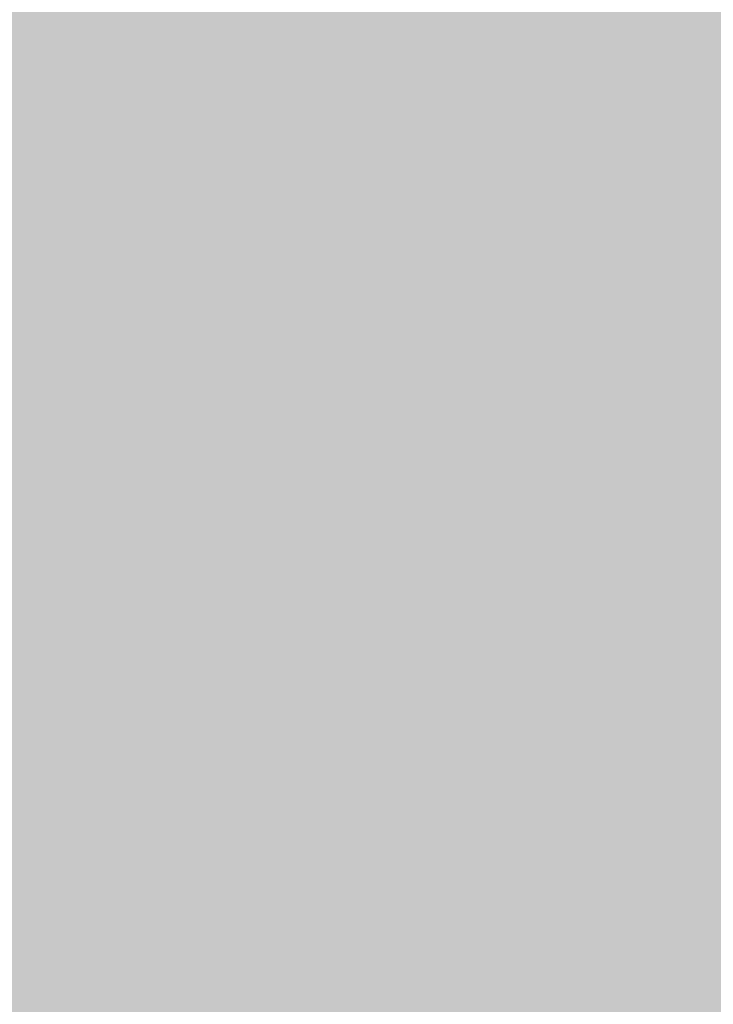
# Model space of a CAD drawing. Units: feet. Extents: x 3168 to 4724, y 827 to 1477.
# Tile 17 of 256: x 3257.497 to 3261.901, y 1087.401 to 1093.654. Entities that reach past the tile are written whole.
import ezdxf

# ---------------------------------------------------------------- set-up
doc = ezdxf.new("R2010")
doc.units = ezdxf.units.FT
doc.layers.add('A-ELEV-PATT', color=8, linetype='Continuous', lineweight=13)

msp = doc.modelspace()

# ---------------------------------------------------------------- hatches: boundary and pattern name
at = {"layer": 'A-ELEV-PATT'}
h = msp.add_hatch(color=256, dxfattribs=at)
h.dxf.hatch_style = 1
edge = h.paths.add_edge_path()
edge.add_ellipse((3552.9058, 979.2201), major_axis=(36.7449, 0), ratio=0.4848485, start_angle=0, end_angle=360)
edge = h.paths.add_edge_path()
edge.add_ellipse((3559.8916, 929.2523), major_axis=(36.7449, 0), ratio=0.4848485, start_angle=0, end_angle=360)
edge = h.paths.add_edge_path()
edge.add_line((3299.3168, 1198.6061), (3479.9167, 1198.6061))
edge.add_line((3479.9167, 1198.6061), (3479.9167, 1209.8686))
edge.add_spline(control_points=[(3479.9167, 1209.8686), (3464.3012, 1209.8686), (3448.6856, 1209.8686), (3410.9491, 1209.8686), (3388.8282, 1209.8686), (3355.6469, 1209.8686), (3344.5864, 1209.8686), (3327.9957, 1209.8686), (3322.4655, 1209.8686), (3314.1702, 1209.8686), (3311.4051, 1209.8686), (3307.2574, 1209.8686), (3305.8748, 1209.8686), (3303.801, 1209.8686), (3303.1097, 1209.8686), (3302.0728, 1209.8686), (3301.7272, 1209.8686), (3301.2087, 1209.8686), (3301.0359, 1209.8686), (3300.7767, 1209.8686), (3300.6903, 1209.8686), (3300.5606, 1209.8686), (3300.5174, 1209.8686), (3300.4526, 1209.8686), (3300.431, 1209.8686), (3300.3986, 1209.8686), (3300.3878, 1209.8686), (3300.3662, 1209.8686), (3300.3457, 1209.8686), (3300.3455, 1209.8686), (3300.3455, 1209.8686), (3300.3433, 1209.8686), (3300.3411, 1209.8686), (3300.3379, 1209.8686), (3300.3368, 1209.8686), (3300.3339, 1209.8686), (3300.3321, 1209.8686), (3300.3255, 1209.8686), (3300.3207, 1209.8686), (3300.3109, 1209.8686), (3300.306, 1209.8686), (3300.2905, 1209.8686), (3300.28, 1209.8686), (3300.2324, 1209.8688), (3300.1953, 1209.869), (3299.9511, 1209.8706), (3299.7448, 1209.8743), (3299.4368, 1209.8833), (3299.3344, 1209.8868), (3299.1811, 1209.8929), (3299.13, 1209.8951), (3298.6522, 1209.9168), (3298.2295, 1209.9457), (3297.6016, 1210.0024), (3297.3934, 1210.0235), (3297.0827, 1210.0583), (3296.9793, 1210.0705), (3296.293, 1210.1549), (3295.7181, 1210.2434), (3294.8687, 1210.3989), (3294.5877, 1210.4545), (3294.1693, 1210.5433), (3294.0304, 1210.5739), (3291.7071, 1211.1012), (3289.6536, 1211.8134), (3285.7763, 1213.564), (3283.9514, 1214.6035), (3280.5122, 1216.9801), (3278.8972, 1218.3176), (3276.3799, 1220.8295), (3275.416, 1221.9177), (3274.0393, 1223.7077), (3273.581, 1224.3495), (3273.1432, 1225.0163)], knot_values=[39.119033, 39.119033, 39.119033, 39.119033, 39.286353, 39.286353, 39.523379, 39.523379, 39.641892, 39.641892, 39.701148, 39.701148, 39.730777, 39.730777, 39.745591, 39.745591, 39.752998, 39.752998, 39.756701, 39.756701, 39.758553, 39.758553, 39.759479, 39.759479, 39.759942, 39.759942, 39.760173, 39.760173, 39.760289, 39.760289, 39.760405, 39.760405, 39.760463, 39.760463, 39.763389, 39.763389, 39.764851, 39.764851, 39.767304, 39.767304, 39.773825, 39.773825, 39.78057, 39.78057, 39.79477, 39.79477, 39.845194, 39.845194, 40.126715, 40.126715, 40.267476, 40.267476, 40.337856, 40.337856, 40.927023, 40.927023, 41.221606, 41.221606, 41.368898, 41.368898, 42.202622, 42.202622, 42.619485, 42.619485, 42.827916, 42.827916, 46.118323, 46.118323, 49.408731, 49.408731, 52.699139, 52.699139, 54.927489, 54.927489, 56.104228, 56.104228, 56.104228, 56.104228], weights=[1, 1, 1, 1, 1, 1, 1, 1, 1, 1, 1, 1, 1, 1, 1, 1, 1, 1, 1, 1, 1, 1, 1, 1, 1, 1, 1, 1, 1, 1, 1, 1, 1, 1, 1, 1, 1, 1, 1, 1, 1, 1, 1, 1, 1, 1, 1, 1, 1, 1, 1, 1, 1, 1, 1, 1, 1, 1, 1, 1, 1, 1, 1, 1, 1, 1, 1, 1, 1, 1, 1, 1, 1, 1], degree=3, periodic=0)
edge.add_line((3273.1432, 1225.0163), (3273.1432, 1099.0163))
edge.add_line((3273.1432, 1099.0163), (3299.3168, 1099.0163))
edge.add_line((3299.3168, 1099.0163), (3299.3168, 1198.6061))
edge = h.paths.add_edge_path()
edge.add_line((3304.7584, 1324.1581), (3479.9167, 1324.1581))
edge.add_line((3479.9167, 1324.1581), (3479.9167, 1335.7146))
edge.add_line((3479.9167, 1335.7146), (3269.1616, 1335.7146))
edge.add_spline(control_points=[(3269.1616, 1335.7146), (3264.0242, 1335.7146), (3258.3641, 1328.9582), (3259.2643, 1323.9003)], knot_values=[0, 0, 0, 0, 15.412191, 15.412191, 15.412191, 15.412191], degree=3, periodic=0)
edge.add_line((3259.2643, 1323.9003), (3265.5168, 1288.7691))
edge.add_line((3265.5168, 1288.7691), (3275.2651, 1261.5456))
edge.add_line((3275.2651, 1261.5456), (3304.7584, 1261.5456))
edge.add_line((3304.7584, 1261.5456), (3304.7584, 1324.1581))
h = msp.add_hatch(color=256, dxfattribs=at)
h.dxf.hatch_style = 1
h.paths.add_polyline_path([(3384.5252, 1099.0163), (3335.0292, 1099.0163), (3299.3168, 1099.0163), (3273.1432, 1099.0163), (3217.5654, 1099.0163), (3168.0693, 827.1163), (3335.0292, 827.1163)])

doc.saveas('drawing.dxf')
